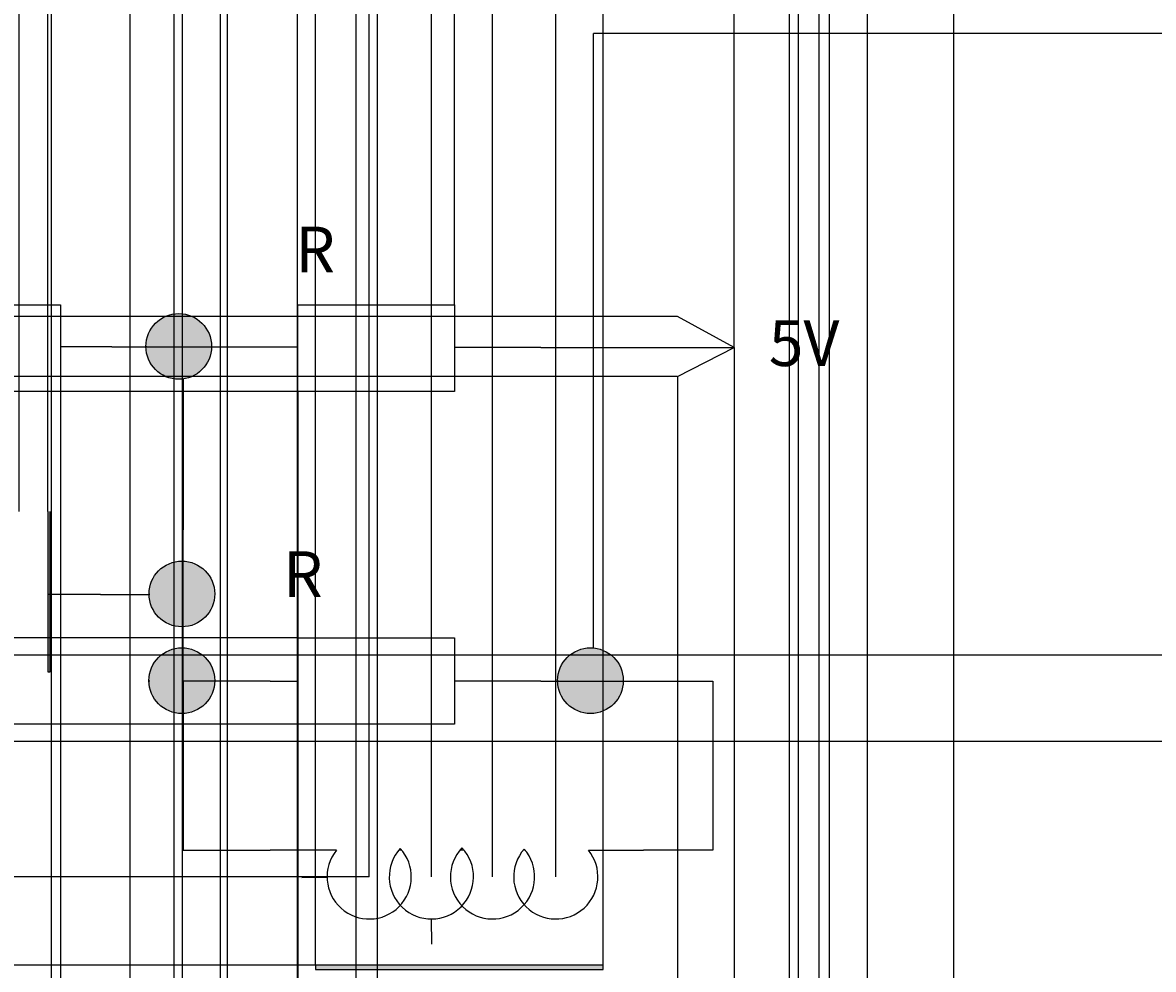
# Model space of a CAD drawing. Units: inches. Extents: x 35362 to 73946, y 43607 to 67532.
# Tile 127 of 134: x 52380 to 57838, y 46109 to 50677. Entities that reach past the tile are written whole.
import ezdxf

# ---------------------------------------------------------------- set-up
doc = ezdxf.new("R2010")
doc.units = ezdxf.units.IN
doc.header["$MEASUREMENT"] = 0
for name, color, linetype, lineweight in [('A-ANNO-DIMS', 2, 'Continuous', 18), ('E-ANNO-TEXT', 5, 'Continuous', 18), ('E-SYMB', 1, 'Continuous', 25), ('E-SYMB-PATT', 1, 'Continuous', 13), ('E-WIRE', 3, 'Continuous', 25)]:
    doc.layers.add(name, color=color, linetype=linetype, lineweight=lineweight)
doc.styles.get("Standard").update_dxf_attribs({"font": 'arial.ttf'})
doc.dimstyles.get("Standard").update_dxf_attribs({"dimtxt": 0.18, "dimasz": 0.18, "dimexe": 0.18, "dimexo": 0.0625, "dimgap": 0.09, "dimtad": 0, "dimtih": 1, "dimtoh": 1, "dimdec": 4, "dimzin": 0, "dimdsep": 46, "dimtxsty": 'Standard', "dimcen": 0.09, "dimadec": 0, "dimazin": 0, "dimtfac": 1, "dimtdec": 4, "dimtofl": 0, "dimtmove": 0, "dimatfit": 3, "dimfxl": 1, "dimtolj": 1, "dimtzin": 0, "dimarcsym": 0})

# ---------------------------------------------------------------- blocks, each defined once
blk = doc.blocks.new('CT-CORE')
for p, q in [((0, 1388), (0, 0)), ((20, 1388), (0, 1388)), ((20, 0), (20, 1388)), ((270.7, 1388), (270.7, 0)), ((290.7, 1388), (270.7, 1388)), ((290.7, 0), (290.7, 1388)), ((659, 1388), (659, 1014.6)), ((679, 1388), (659, 1388)), ((679, 1015.4), (679, 1388)), ((659, 544.4), (659, 0)), ((679, 0), (679, 543.5)), ((0, 0), (20, 0)), ((270.7, 0), (290.7, 0)), ((659, 0), (679, 0))]:
    blk.add_line(p, q)
blk.add_arc((679, 779.5), 235.9, 90, 270)
blk = doc.blocks.new('PWR-5V')
for p, q in [((149.8, 1350.9), (0, 1075.9)), ((149.8, 833.1), (149.8, 1350.9)), ((290, 1075.9), (149.8, 1350.9)), ((149.8, 416.3), (149.8, 833.1)), ((149.8, 416.3), (149.8, 0))]:
    blk.add_line(p, q)
blk = doc.blocks.new('*D5')
at = {"layer": 'A-ANNO-DIMS', "color": 0, "lineweight": -2, "transparency": 16777216}
for p, q in [((37121.9, 46919.3), (37121.9, 43606.7)), ((69871.5, 45449.8), (69871.5, 43606.7)), ((37122.1, 43606.9), (53496.3, 43606.9)), ((69871.3, 43606.9), (53497.2, 43606.9))]:
    blk.add_line(p, q, dxfattribs=at)
at = {"layer": 'A-ANNO-DIMS', "color": 0, "transparency": 16777216}
for points in [[(37122.1, 43606.9), (37122.1, 43606.8), (37121.9, 43606.9)], [(69871.3, 43606.9), (69871.3, 43606.8), (69871.5, 43606.9)]]:
    blk.add_solid(points, dxfattribs=at)
at = {"layer": 'Defpoints', "color": 0, "transparency": 16777216}
for p in [(37121.9, 46919.4), (69871.5, 45449.9), (69871.5, 43606.9)]:
    blk.add_point(p, dxfattribs=at)
at = {"layer": 'A-ANNO-DIMS', "color": 0, "transparency": 16777216, "insert": (53496.7, 43606.9), "char_height": 0.18, "attachment_point": 5}
blk.add_mtext('\\A1;32750', dxfattribs=at)
blk = doc.blocks.new('*D11')
at = {"layer": 'A-ANNO-DIMS', "color": 0, "lineweight": -2, "transparency": 16777216}
for p, q in [((47978.7, 56028.8), (47978.7, 43606.7)), ((53109.8, 56028.8), (53109.8, 43606.7)), ((47978.8, 43606.9), (50543.9, 43606.9)), ((53109.6, 43606.9), (50544.6, 43606.9))]:
    blk.add_line(p, q, dxfattribs=at)
at = {"layer": 'A-ANNO-DIMS', "color": 0, "transparency": 16777216}
for points in [[(47978.8, 43606.9), (47978.8, 43606.8), (47978.7, 43606.9)], [(53109.6, 43606.9), (53109.6, 43606.8), (53109.8, 43606.9)]]:
    blk.add_solid(points, dxfattribs=at)
at = {"layer": 'Defpoints', "color": 0, "transparency": 16777216}
for p in [(47978.7, 56028.8), (53109.8, 56028.8), (53109.8, 43606.9)]:
    blk.add_point(p, dxfattribs=at)
at = {"layer": 'A-ANNO-DIMS', "color": 0, "transparency": 16777216, "insert": (50544.2, 43606.9), "char_height": 0.18, "attachment_point": 5}
blk.add_mtext('\\A1;5131', dxfattribs=at)
blk = doc.blocks.new('*D23')
at = {"layer": 'A-ANNO-DIMS', "color": 0, "lineweight": -2, "transparency": 16777216}
for p, q in [((53727.6, 46552.2), (53849.4, 46553.3)), ((54052.8, 46555.3), (54053, 46555.3)), ((54052.9, 46555.2), (54052.9, 46555.4))]:
    blk.add_line(p, q, dxfattribs=at)
at = {"layer": 'A-ANNO-DIMS', "color": 0, "transparency": 16777216}
blk.add_solid([(53849.4, 46553.4), (53849.4, 46553.3), (53849.6, 46553.3)], dxfattribs=at)
at = {"layer": 'Defpoints', "color": 0, "transparency": 16777216}
for p in [(53849.6, 46553.3), (54052.9, 46555.3)]:
    blk.add_point(p, dxfattribs=at)
at = {"layer": 'A-ANNO-DIMS', "color": 0, "transparency": 16777216, "insert": (53726.8, 46552.2), "char_height": 0.18, "attachment_point": 5}
blk.add_mtext('\\A1;20X R203.33', dxfattribs=at)
blk = doc.blocks.new('*D39')
at = {"layer": 'A-ANNO-DIMS', "color": 0, "lineweight": -2, "transparency": 16777216}
for p, q in [((53793.6, 46128.9), (53793.6, 67531.7)), ((53793.8, 67531.5), (54487.2, 67531.5)), ((55181.5, 67531.5), (54488.1, 67531.5)), ((55181.6, 46128.9), (55181.6, 67531.7))]:
    blk.add_line(p, q, dxfattribs=at)
at = {"layer": 'A-ANNO-DIMS', "color": 0, "transparency": 16777216}
for points in [[(53793.8, 67531.5), (53793.8, 67531.5), (53793.6, 67531.5)], [(55181.5, 67531.5), (55181.5, 67531.5), (55181.6, 67531.5)]]:
    blk.add_solid(points, dxfattribs=at)
at = {"layer": 'Defpoints', "color": 0, "transparency": 16777216}
for p in [(55181.6, 67531.5), (53793.6, 46128.9), (55181.6, 46128.9)]:
    blk.add_point(p, dxfattribs=at)
at = {"layer": 'A-ANNO-DIMS', "color": 0, "transparency": 16777216, "insert": (54487.6, 67531.5), "char_height": 0.18, "attachment_point": 5}
blk.add_mtext('\\A1;1388.0', dxfattribs=at)
blk = doc.blocks.new('*D40')
at = {"layer": 'A-ANNO-DIMS', "color": 0, "lineweight": -2, "transparency": 16777216}
for p, q in [((56873.5, 53351.5), (35361.8, 53351.5)), ((35361.9, 53351.3), (35361.9, 51333.3)), ((35361.9, 49314.8), (35361.9, 51332.9)), ((51806.5, 49314.7), (35361.8, 49314.7))]:
    blk.add_line(p, q, dxfattribs=at)
at = {"layer": 'A-ANNO-DIMS', "color": 0, "transparency": 16777216}
for points in [[(35361.9, 53351.3), (35362, 53351.3), (35361.9, 53351.5)], [(35361.9, 49314.8), (35362, 49314.8), (35361.9, 49314.7)]]:
    blk.add_solid(points, dxfattribs=at)
at = {"layer": 'Defpoints', "color": 0, "transparency": 16777216}
for p in [(35361.9, 53351.5), (56873.6, 53351.5), (51806.5, 49314.7)]:
    blk.add_point(p, dxfattribs=at)
at = {"layer": 'A-ANNO-DIMS', "color": 0, "transparency": 16777216, "insert": (35361.9, 51333.1), "char_height": 0.18, "attachment_point": 5}
blk.add_mtext('\\A1;4036.9', dxfattribs=at)
blk = doc.blocks.new('*D43')
at = {"layer": 'A-ANNO-DIMS', "color": 0, "lineweight": -2, "transparency": 16777216}
for p, q in [((62004.7, 47625.2), (35361.8, 47625.2)), ((35361.9, 47625), (35361.9, 47416.9)), ((35361.9, 47208.4), (35361.9, 47416.5)), ((62004.7, 47208.2), (35361.8, 47208.2))]:
    blk.add_line(p, q, dxfattribs=at)
at = {"layer": 'A-ANNO-DIMS', "color": 0, "transparency": 16777216}
for points in [[(35361.9, 47625), (35362, 47625), (35361.9, 47625.2)], [(35361.9, 47208.4), (35362, 47208.4), (35361.9, 47208.2)]]:
    blk.add_solid(points, dxfattribs=at)
at = {"layer": 'Defpoints', "color": 0, "transparency": 16777216}
for p in [(62004.7, 47625.2), (35361.9, 47208.2), (62004.7, 47208.2)]:
    blk.add_point(p, dxfattribs=at)
at = {"layer": 'A-ANNO-DIMS', "color": 0, "transparency": 16777216, "insert": (35361.9, 47416.7), "char_height": 0.18, "attachment_point": 5}
blk.add_mtext('\\A1;416.9', dxfattribs=at)
blk = doc.blocks.new('*D44')
at = {"layer": 'A-ANNO-DIMS', "color": 0, "lineweight": -2, "transparency": 16777216}
for p, q in [((52517.8, 64828.5), (52517.8, 43606.7)), ((54090.8, 64828.5), (54090.8, 43606.7)), ((52518, 43606.9), (53303.8, 43606.9)), ((54090.6, 43606.9), (53304.7, 43606.9))]:
    blk.add_line(p, q, dxfattribs=at)
at = {"layer": 'A-ANNO-DIMS', "color": 0, "transparency": 16777216}
for points in [[(52518, 43606.9), (52518, 43606.8), (52517.8, 43606.9)], [(54090.6, 43606.9), (54090.6, 43606.8), (54090.8, 43606.9)]]:
    blk.add_solid(points, dxfattribs=at)
at = {"layer": 'Defpoints', "color": 0, "transparency": 16777216}
for p in [(52517.8, 64828.6), (54090.8, 64828.6), (54090.8, 43606.9)]:
    blk.add_point(p, dxfattribs=at)
at = {"layer": 'A-ANNO-DIMS', "color": 0, "transparency": 16777216, "insert": (53304.3, 43606.9), "char_height": 0.18, "attachment_point": 5}
blk.add_mtext('\\A1;1573.0', dxfattribs=at)
blk = doc.blocks.new('*D49')
at = {"layer": 'A-ANNO-DIMS', "color": 0, "lineweight": -2, "transparency": 16777216}
for p, q in [((56457.3, 54249.8), (56457.3, 43606.7)), ((56873.6, 54249.8), (56873.6, 43606.7)), ((56457.5, 43606.9), (56665, 43606.9)), ((56873.4, 43606.9), (56665.8, 43606.9))]:
    blk.add_line(p, q, dxfattribs=at)
at = {"layer": 'A-ANNO-DIMS', "color": 0, "transparency": 16777216}
for points in [[(56457.5, 43606.9), (56457.5, 43606.8), (56457.3, 43606.9)], [(56873.4, 43606.9), (56873.4, 43606.8), (56873.6, 43606.9)]]:
    blk.add_solid(points, dxfattribs=at)
at = {"layer": 'Defpoints', "color": 0, "transparency": 16777216}
for p in [(56457.3, 54249.8), (56873.6, 54249.8), (56873.6, 43606.9)]:
    blk.add_point(p, dxfattribs=at)
at = {"layer": 'A-ANNO-DIMS', "color": 0, "transparency": 16777216, "insert": (56665.4, 43606.9), "char_height": 0.18, "attachment_point": 5}
blk.add_mtext('\\A1;416.3', dxfattribs=at)
blk = doc.blocks.new('*D53')
at = {"layer": 'A-ANNO-DIMS', "color": 0, "lineweight": -2, "transparency": 16777216}
for p, q in [((56873.6, 53351.5), (56873.6, 43606.7)), ((58224.8, 52935.2), (58224.8, 43606.7)), ((56873.8, 43606.9), (57548.7, 43606.9)), ((58224.6, 43606.9), (57549.6, 43606.9))]:
    blk.add_line(p, q, dxfattribs=at)
at = {"layer": 'A-ANNO-DIMS', "color": 0, "transparency": 16777216}
for points in [[(56873.8, 43606.9), (56873.8, 43606.8), (56873.6, 43606.9)], [(58224.6, 43606.9), (58224.6, 43606.8), (58224.8, 43606.9)]]:
    blk.add_solid(points, dxfattribs=at)
at = {"layer": 'Defpoints', "color": 0, "transparency": 16777216}
for p in [(56873.6, 53351.5), (58224.8, 52935.2), (58224.8, 43606.9)]:
    blk.add_point(p, dxfattribs=at)
at = {"layer": 'A-ANNO-DIMS', "color": 0, "transparency": 16777216, "insert": (57549.2, 43606.9), "char_height": 0.18, "attachment_point": 5}
blk.add_mtext('\\A1;1351.2', dxfattribs=at)
blk = doc.blocks.new('*D63')
at = {"layer": 'A-ANNO-DIMS', "color": 0, "lineweight": -2, "transparency": 16777216}
for p, q in [((53727.6, 46552.2), (53849.4, 46553.3)), ((54052.8, 46555.3), (54053, 46555.3)), ((54052.9, 46555.2), (54052.9, 46555.4))]:
    blk.add_line(p, q, dxfattribs=at)
at = {"layer": 'A-ANNO-DIMS', "color": 0, "transparency": 16777216}
blk.add_solid([(53849.4, 46553.4), (53849.4, 46553.3), (53849.6, 46553.3)], dxfattribs=at)
at = {"layer": 'Defpoints', "color": 0, "transparency": 16777216}
for p in [(53849.6, 46553.3), (54052.9, 46555.3)]:
    blk.add_point(p, dxfattribs=at)
at = {"layer": 'A-ANNO-DIMS', "color": 0, "transparency": 16777216, "insert": (53726.8, 46552.2), "char_height": 0.18, "attachment_point": 5}
blk.add_mtext('\\A1;20X R203.33', dxfattribs=at)
blk = doc.blocks.new('*D67')
at = {"layer": 'A-ANNO-DIMS', "color": 0, "lineweight": -2, "transparency": 16777216}
for p, q in [((56873.5, 53351.5), (35361.8, 53351.5)), ((35361.9, 53351.3), (35361.9, 49400.9)), ((35361.9, 45450.1), (35361.9, 49400.5)), ((53793.6, 45449.9), (35361.8, 45449.9))]:
    blk.add_line(p, q, dxfattribs=at)
at = {"layer": 'A-ANNO-DIMS', "color": 0, "transparency": 16777216}
for points in [[(35361.9, 53351.3), (35362, 53351.3), (35361.9, 53351.5)], [(35361.9, 45450.1), (35362, 45450.1), (35361.9, 45449.9)]]:
    blk.add_solid(points, dxfattribs=at)
at = {"layer": 'Defpoints', "color": 0, "transparency": 16777216}
for p in [(35361.9, 53351.5), (56873.6, 53351.5), (53793.6, 45449.9)]:
    blk.add_point(p, dxfattribs=at)
at = {"layer": 'A-ANNO-DIMS', "color": 0, "transparency": 16777216, "insert": (35361.9, 49400.7), "char_height": 0.18, "attachment_point": 5}
blk.add_mtext('\\A1;7901.6', dxfattribs=at)
blk = doc.blocks.new('*D76')
at = {"layer": 'A-ANNO-DIMS', "color": 0, "lineweight": -2, "transparency": 16777216}
for p, q in [((54052.8, 46555.3), (35361.8, 46555.3)), ((35361.9, 46555.1), (35361.9, 46342.3)), ((35361.9, 46129.1), (35361.9, 46341.9)), ((53793.6, 46128.9), (35361.8, 46128.9))]:
    blk.add_line(p, q, dxfattribs=at)
at = {"layer": 'A-ANNO-DIMS', "color": 0, "transparency": 16777216}
for points in [[(35361.9, 46555.1), (35362, 46555.1), (35361.9, 46555.3)], [(35361.9, 46129.1), (35362, 46129.1), (35361.9, 46128.9)]]:
    blk.add_solid(points, dxfattribs=at)
at = {"layer": 'Defpoints', "color": 0, "transparency": 16777216}
for p in [(35361.9, 46555.3), (54052.9, 46555.3), (53793.6, 46128.9)]:
    blk.add_point(p, dxfattribs=at)
at = {"layer": 'A-ANNO-DIMS', "color": 0, "transparency": 16777216, "insert": (35361.9, 46342.1), "char_height": 0.18, "attachment_point": 5}
blk.add_mtext('\\A1;426.4', dxfattribs=at)
blk = doc.blocks.new('*D77')
at = {"layer": 'A-ANNO-DIMS', "color": 0, "lineweight": -2, "transparency": 16777216}
for p, q in [((53793.6, 46128.9), (53793.6, 67531.7)), ((53793.8, 67531.5), (53922.8, 67531.5)), ((54052.7, 67531.5), (53923.7, 67531.5)), ((54052.9, 46555.4), (54052.9, 67531.7))]:
    blk.add_line(p, q, dxfattribs=at)
at = {"layer": 'A-ANNO-DIMS', "color": 0, "transparency": 16777216}
for points in [[(53793.8, 67531.5), (53793.8, 67531.5), (53793.6, 67531.5)], [(54052.7, 67531.5), (54052.7, 67531.5), (54052.9, 67531.5)]]:
    blk.add_solid(points, dxfattribs=at)
at = {"layer": 'Defpoints', "color": 0, "transparency": 16777216}
for p in [(54052.9, 67531.5), (54052.9, 46555.3), (53793.6, 46128.9)]:
    blk.add_point(p, dxfattribs=at)
at = {"layer": 'A-ANNO-DIMS', "color": 0, "transparency": 16777216, "insert": (53923.3, 67531.5), "char_height": 0.18, "attachment_point": 5}
blk.add_mtext('\\A1;259.26', dxfattribs=at)
blk = doc.blocks.new('*D78')
at = {"layer": 'A-ANNO-DIMS', "color": 0, "lineweight": -2, "transparency": 16777216}
for p, q in [((54052.9, 46555.4), (54052.9, 67531.7)), ((54053.1, 67531.5), (54202.6, 67531.5)), ((54352.9, 67531.5), (54203.4, 67531.5)), ((54353.1, 46555.4), (54353.1, 67531.7))]:
    blk.add_line(p, q, dxfattribs=at)
at = {"layer": 'A-ANNO-DIMS', "color": 0, "transparency": 16777216}
for points in [[(54053.1, 67531.5), (54053.1, 67531.5), (54052.9, 67531.5)], [(54352.9, 67531.5), (54352.9, 67531.5), (54353.1, 67531.5)]]:
    blk.add_solid(points, dxfattribs=at)
at = {"layer": 'Defpoints', "color": 0, "transparency": 16777216}
for p in [(54353.1, 67531.5), (54052.9, 46555.3), (54353.1, 46555.3)]:
    blk.add_point(p, dxfattribs=at)
at = {"layer": 'A-ANNO-DIMS', "color": 0, "transparency": 16777216, "insert": (54203, 67531.5), "char_height": 0.18, "attachment_point": 5}
blk.add_mtext('\\A1;300.2', dxfattribs=at)
blk = doc.blocks.new('*D79')
at = {"layer": 'A-ANNO-DIMS', "color": 0, "lineweight": -2, "transparency": 16777216}
for p, q in [((54353.1, 46555.4), (54353.1, 67531.7)), ((54353.3, 67531.5), (54500.2, 67531.5)), ((54648, 67531.5), (54501, 67531.5)), ((54648.2, 46555.4), (54648.2, 67531.7))]:
    blk.add_line(p, q, dxfattribs=at)
at = {"layer": 'A-ANNO-DIMS', "color": 0, "transparency": 16777216}
for points in [[(54353.3, 67531.5), (54353.3, 67531.5), (54353.1, 67531.5)], [(54648, 67531.5), (54648, 67531.5), (54648.2, 67531.5)]]:
    blk.add_solid(points, dxfattribs=at)
at = {"layer": 'Defpoints', "color": 0, "transparency": 16777216}
for p in [(54648.2, 67531.5), (54353.1, 46555.3), (54648.2, 46555.3)]:
    blk.add_point(p, dxfattribs=at)
at = {"layer": 'A-ANNO-DIMS', "color": 0, "transparency": 16777216, "insert": (54500.6, 67531.5), "char_height": 0.18, "attachment_point": 5}
blk.add_mtext('\\A1;295.1', dxfattribs=at)
blk = doc.blocks.new('*D80')
at = {"layer": 'A-ANNO-DIMS', "color": 0, "lineweight": -2, "transparency": 16777216}
for p, q in [((54648.2, 46555.4), (54648.2, 67531.7)), ((54648.4, 67531.5), (54800.3, 67531.5)), ((54953.3, 67531.5), (54801.3, 67531.5)), ((54953.4, 46555.4), (54953.4, 67531.7))]:
    blk.add_line(p, q, dxfattribs=at)
at = {"layer": 'A-ANNO-DIMS', "color": 0, "transparency": 16777216}
for points in [[(54648.4, 67531.5), (54648.4, 67531.5), (54648.2, 67531.5)], [(54953.3, 67531.5), (54953.3, 67531.5), (54953.4, 67531.5)]]:
    blk.add_solid(points, dxfattribs=at)
at = {"layer": 'Defpoints', "color": 0, "transparency": 16777216}
for p in [(54953.4, 67531.5), (54648.2, 46555.3), (54953.4, 46555.3)]:
    blk.add_point(p, dxfattribs=at)
at = {"layer": 'A-ANNO-DIMS', "color": 0, "transparency": 16777216, "insert": (54800.8, 67531.5), "char_height": 0.18, "attachment_point": 5}
blk.add_mtext('\\A1;305.27', dxfattribs=at)
blk = doc.blocks.new('*D82')
at = {"layer": 'A-ANNO-DIMS', "color": 0, "lineweight": -2, "transparency": 16777216}
for p, q in [((54464.4, 49314.7), (54464.4, 67531.7)), ((54464.6, 67531.5), (55139.4, 67531.5)), ((55815.1, 67531.5), (55140.3, 67531.5)), ((55815.3, 49110.2), (55815.3, 67531.7))]:
    blk.add_line(p, q, dxfattribs=at)
at = {"layer": 'A-ANNO-DIMS', "color": 0, "transparency": 16777216}
for points in [[(54464.6, 67531.5), (54464.6, 67531.5), (54464.4, 67531.5)], [(55815.1, 67531.5), (55815.1, 67531.5), (55815.3, 67531.5)]]:
    blk.add_solid(points, dxfattribs=at)
at = {"layer": 'Defpoints', "color": 0, "transparency": 16777216}
for p in [(55815.3, 67531.5), (54464.4, 49314.7), (55815.3, 49110.1)]:
    blk.add_point(p, dxfattribs=at)
at = {"layer": 'A-ANNO-DIMS', "color": 0, "transparency": 16777216, "insert": (55139.9, 67531.5), "char_height": 0.18, "attachment_point": 5}
blk.add_mtext('\\A1;1350.9', dxfattribs=at)
blk = doc.blocks.new('*D83')
at = {"layer": 'A-ANNO-DIMS', "color": 0, "lineweight": -2, "transparency": 16777216}
for p, q in [((55815.3, 49110), (55815.3, 43606.7)), ((55540.3, 48969.9), (55540.3, 43606.7)), ((55540.5, 43606.9), (55677.4, 43606.9)), ((55815.1, 43606.9), (55678.2, 43606.9))]:
    blk.add_line(p, q, dxfattribs=at)
at = {"layer": 'A-ANNO-DIMS', "color": 0, "transparency": 16777216}
for points in [[(55540.5, 43606.9), (55540.5, 43606.8), (55540.3, 43606.9)], [(55815.1, 43606.9), (55815.1, 43606.8), (55815.3, 43606.9)]]:
    blk.add_solid(points, dxfattribs=at)
at = {"layer": 'Defpoints', "color": 0, "transparency": 16777216}
for p in [(55815.3, 49110.1), (55540.3, 48970), (55815.3, 43606.9)]:
    blk.add_point(p, dxfattribs=at)
at = {"layer": 'A-ANNO-DIMS', "color": 0, "transparency": 16777216, "insert": (55677.8, 43606.9), "char_height": 0.18, "attachment_point": 5}
blk.add_mtext('\\A1;275.0', dxfattribs=at)
blk = doc.blocks.new('*D84')
at = {"layer": 'A-ANNO-DIMS', "color": 0, "lineweight": -2, "transparency": 16777216}
for p, q in [((55540.2, 49259.9), (35361.8, 49259.9)), ((35361.9, 49259.8), (35361.9, 49115.1)), ((35361.9, 48970.2), (35361.9, 49114.8)), ((55540.2, 48970), (35361.8, 48970))]:
    blk.add_line(p, q, dxfattribs=at)
at = {"layer": 'A-ANNO-DIMS', "color": 0, "transparency": 16777216}
for points in [[(35361.9, 49259.8), (35362, 49259.8), (35361.9, 49259.9)], [(35361.9, 48970.2), (35362, 48970.2), (35361.9, 48970)]]:
    blk.add_solid(points, dxfattribs=at)
at = {"layer": 'Defpoints', "color": 0, "transparency": 16777216}
for p in [(35361.9, 49259.9), (55540.3, 49259.9), (55540.3, 48970)]:
    blk.add_point(p, dxfattribs=at)
at = {"layer": 'A-ANNO-DIMS', "color": 0, "transparency": 16777216, "insert": (35361.9, 49115), "char_height": 0.18, "attachment_point": 5}
blk.add_mtext('\\A1;289.96', dxfattribs=at)
blk = doc.blocks.new('*D88')
at = {"layer": 'A-ANNO-DIMS', "color": 0, "lineweight": -2, "transparency": 16777216}
for p, q in [((52362.6, 48318.3), (52362.6, 67531.7)), ((52362.7, 67531.5), (52432.1, 67531.5)), ((52502.2, 67531.5), (52432.8, 67531.5)), ((52502.4, 48318.3), (52502.4, 67531.7))]:
    blk.add_line(p, q, dxfattribs=at)
at = {"layer": 'A-ANNO-DIMS', "color": 0, "transparency": 16777216}
for points in [[(52362.7, 67531.5), (52362.7, 67531.5), (52362.6, 67531.5)], [(52502.2, 67531.5), (52502.2, 67531.5), (52502.4, 67531.5)]]:
    blk.add_solid(points, dxfattribs=at)
at = {"layer": 'Defpoints', "color": 0, "transparency": 16777216}
for p in [(52502.4, 67531.5), (52362.6, 48318.3), (52502.4, 48318.3)]:
    blk.add_point(p, dxfattribs=at)
at = {"layer": 'A-ANNO-DIMS', "color": 0, "transparency": 16777216, "insert": (52432.5, 67531.5), "char_height": 0.18, "attachment_point": 5}
blk.add_mtext('\\A1;139.8', dxfattribs=at)
blk = doc.blocks.new('*D89')
at = {"layer": 'A-ANNO-DIMS', "color": 0, "lineweight": -2, "transparency": 16777216}
for p, q in [((53707.7, 48897.7), (35361.8, 48897.7)), ((35361.9, 48897.6), (35361.9, 48303.2)), ((35361.9, 47708.4), (35361.9, 48302.8)), ((53707.7, 47708.2), (35361.8, 47708.2))]:
    blk.add_line(p, q, dxfattribs=at)
at = {"layer": 'A-ANNO-DIMS', "color": 0, "transparency": 16777216}
for points in [[(35361.9, 48897.6), (35362, 48897.6), (35361.9, 48897.7)], [(35361.9, 47708.4), (35362, 47708.4), (35361.9, 47708.2)]]:
    blk.add_solid(points, dxfattribs=at)
at = {"layer": 'Defpoints', "color": 0, "transparency": 16777216}
for p in [(53707.8, 48897.7), (35361.9, 47708.2), (53707.8, 47708.2)]:
    blk.add_point(p, dxfattribs=at)
at = {"layer": 'A-ANNO-DIMS', "color": 0, "transparency": 16777216, "insert": (35361.9, 48303), "char_height": 0.18, "attachment_point": 5}
blk.add_mtext('\\A1;1189.5', dxfattribs=at)
blk = doc.blocks.new('*D90')
at = {"layer": 'A-ANNO-DIMS', "color": 0, "lineweight": -2, "transparency": 16777216}
for p, q in [((53707.7, 47291.3), (35361.8, 47291.3)), ((35361.9, 47291.1), (35361.9, 46710.3)), ((35361.9, 46129.1), (35361.9, 46709.9)), ((53793.6, 46128.9), (35361.8, 46128.9))]:
    blk.add_line(p, q, dxfattribs=at)
at = {"layer": 'A-ANNO-DIMS', "color": 0, "transparency": 16777216}
for points in [[(35361.9, 47291.1), (35362, 47291.1), (35361.9, 47291.3)], [(35361.9, 46129.1), (35362, 46129.1), (35361.9, 46128.9)]]:
    blk.add_solid(points, dxfattribs=at)
at = {"layer": 'Defpoints', "color": 0, "transparency": 16777216}
for p in [(53707.8, 47291.3), (35361.9, 46128.9), (53793.6, 46128.9)]:
    blk.add_point(p, dxfattribs=at)
at = {"layer": 'A-ANNO-DIMS', "color": 0, "transparency": 16777216, "insert": (35361.9, 46710.1), "char_height": 0.18, "attachment_point": 5}
blk.add_mtext('\\A1;1162.4', dxfattribs=at)
blk = doc.blocks.new('*D91')
at = {"layer": 'A-ANNO-DIMS', "color": 0, "lineweight": -2, "transparency": 16777216}
for p, q in [((52563.1, 48897.7), (52563.1, 43606.7)), ((53707.8, 48897.7), (53707.8, 43606.7)), ((52563.3, 43606.9), (53135, 43606.9)), ((53707.6, 43606.9), (53135.9, 43606.9))]:
    blk.add_line(p, q, dxfattribs=at)
at = {"layer": 'A-ANNO-DIMS', "color": 0, "transparency": 16777216}
for points in [[(52563.3, 43606.9), (52563.3, 43606.8), (52563.1, 43606.9)], [(53707.6, 43606.9), (53707.6, 43606.8), (53707.8, 43606.9)]]:
    blk.add_solid(points, dxfattribs=at)
at = {"layer": 'Defpoints', "color": 0, "transparency": 16777216}
for p in [(52563.1, 48897.7), (53707.8, 48897.7), (53707.8, 43606.9)]:
    blk.add_point(p, dxfattribs=at)
at = {"layer": 'A-ANNO-DIMS', "color": 0, "transparency": 16777216, "insert": (53135.5, 43606.9), "char_height": 0.18, "attachment_point": 5}
blk.add_mtext('\\A1;1144.6', dxfattribs=at)
blk = doc.blocks.new('*D96')
at = {"layer": 'A-ANNO-DIMS', "color": 0, "lineweight": -2, "transparency": 16777216}
for p, q in [((53366.8, 64997.6), (53366.8, 43606.7)), ((53988.6, 64997.6), (53988.6, 43606.7)), ((53366.9, 43606.9), (53677.3, 43606.9)), ((53988.4, 43606.9), (53678.1, 43606.9))]:
    blk.add_line(p, q, dxfattribs=at)
at = {"layer": 'A-ANNO-DIMS', "color": 0, "transparency": 16777216}
for points in [[(53366.9, 43606.9), (53366.9, 43606.8), (53366.8, 43606.9)], [(53988.4, 43606.9), (53988.4, 43606.8), (53988.6, 43606.9)]]:
    blk.add_solid(points, dxfattribs=at)
at = {"layer": 'Defpoints', "color": 0, "transparency": 16777216}
for p in [(53366.8, 64997.7), (53988.6, 64997.7), (53988.6, 43606.9)]:
    blk.add_point(p, dxfattribs=at)
at = {"layer": 'A-ANNO-DIMS', "color": 0, "transparency": 16777216, "insert": (53677.7, 43606.9), "char_height": 0.18, "attachment_point": 5}
blk.add_mtext('\\A1;621.8', dxfattribs=at)
blk = doc.blocks.new('*D99')
at = {"layer": 'A-ANNO-DIMS', "color": 0, "lineweight": -2, "transparency": 16777216}
for p, q in [((52897.5, 65291.5), (52897.5, 43606.7)), ((52517.8, 64828.5), (52517.8, 43606.7)), ((52518, 43606.9), (52707.2, 43606.9)), ((52897.3, 43606.9), (52708, 43606.9))]:
    blk.add_line(p, q, dxfattribs=at)
at = {"layer": 'A-ANNO-DIMS', "color": 0, "transparency": 16777216}
for points in [[(52518, 43606.9), (52518, 43606.8), (52517.8, 43606.9)], [(52897.3, 43606.9), (52897.3, 43606.8), (52897.5, 43606.9)]]:
    blk.add_solid(points, dxfattribs=at)
at = {"layer": 'Defpoints', "color": 0, "transparency": 16777216}
for p in [(52897.5, 65291.6), (52517.8, 64828.6), (52897.5, 43606.9)]:
    blk.add_point(p, dxfattribs=at)
at = {"layer": 'A-ANNO-DIMS', "color": 0, "transparency": 16777216, "insert": (52707.6, 43606.9), "char_height": 0.18, "attachment_point": 5}
blk.add_mtext('\\A1;379.7', dxfattribs=at)
blk = doc.blocks.new('*D100')
at = {"layer": 'A-ANNO-DIMS', "color": 0, "lineweight": -2, "transparency": 16777216}
for p, q in [((52897.5, 65291.5), (52897.5, 43606.7)), ((53150.7, 64926.1), (53150.7, 43606.7)), ((52897.7, 43606.9), (53023.7, 43606.9)), ((53150.5, 43606.9), (53024.5, 43606.9))]:
    blk.add_line(p, q, dxfattribs=at)
at = {"layer": 'A-ANNO-DIMS', "color": 0, "transparency": 16777216}
for points in [[(52897.7, 43606.9), (52897.7, 43606.8), (52897.5, 43606.9)], [(53150.5, 43606.9), (53150.5, 43606.8), (53150.7, 43606.9)]]:
    blk.add_solid(points, dxfattribs=at)
at = {"layer": 'Defpoints', "color": 0, "transparency": 16777216}
for p in [(52897.5, 65291.6), (53150.7, 64926.1), (53150.7, 43606.9)]:
    blk.add_point(p, dxfattribs=at)
at = {"layer": 'A-ANNO-DIMS', "color": 0, "transparency": 16777216, "insert": (53024.1, 43606.9), "char_height": 0.18, "attachment_point": 5}
blk.add_mtext('\\A1;253.2', dxfattribs=at)
blk = doc.blocks.new('*D102')
at = {"layer": 'A-ANNO-DIMS', "color": 0, "lineweight": -2, "transparency": 16777216}
for p, q in [((56080.5, 63694.7), (56080.5, 43606.7)), ((56272.5, 63696.8), (56272.5, 43606.7)), ((56080.7, 43606.9), (56176, 43606.9)), ((56272.3, 43606.9), (56176.9, 43606.9))]:
    blk.add_line(p, q, dxfattribs=at)
at = {"layer": 'A-ANNO-DIMS', "color": 0, "transparency": 16777216}
for points in [[(56080.7, 43606.9), (56080.7, 43606.8), (56080.5, 43606.9)], [(56272.3, 43606.9), (56272.3, 43606.8), (56272.5, 43606.9)]]:
    blk.add_solid(points, dxfattribs=at)
at = {"layer": 'Defpoints', "color": 0, "transparency": 16777216}
for p in [(56080.5, 63694.8), (56272.5, 63696.9), (56272.5, 43606.9)]:
    blk.add_point(p, dxfattribs=at)
at = {"layer": 'A-ANNO-DIMS', "color": 0, "transparency": 16777216, "insert": (56176.5, 43606.9), "char_height": 0.18, "attachment_point": 5}
blk.add_mtext('\\A1;191.98', dxfattribs=at)
blk = doc.blocks.new('*D104')
at = {"layer": 'A-ANNO-DIMS', "color": 0, "lineweight": -2, "transparency": 16777216}
for p, q in [((56123.2, 63318.1), (56123.2, 43606.7)), ((56223, 63318.1), (56223, 43606.7)), ((56123.4, 43606.9), (56172.7, 43606.9)), ((56222.8, 43606.9), (56173.5, 43606.9))]:
    blk.add_line(p, q, dxfattribs=at)
at = {"layer": 'A-ANNO-DIMS', "color": 0, "transparency": 16777216}
for points in [[(56123.4, 43606.9), (56123.4, 43606.8), (56123.2, 43606.9)], [(56222.8, 43606.9), (56222.8, 43606.8), (56223, 43606.9)]]:
    blk.add_solid(points, dxfattribs=at)
at = {"layer": 'Defpoints', "color": 0, "transparency": 16777216}
for p in [(56123.2, 63318.1), (56223, 63318.1), (56223, 43606.9)]:
    blk.add_point(p, dxfattribs=at)
at = {"layer": 'A-ANNO-DIMS', "color": 0, "transparency": 16777216, "insert": (56173.1, 43606.9), "char_height": 0.18, "attachment_point": 5}
blk.add_mtext('\\A1;99.74', dxfattribs=at)
blk = doc.blocks.new('*D112')
at = {"layer": 'A-ANNO-DIMS', "color": 0, "lineweight": -2, "transparency": 16777216}
for p, q in [((53332.8, 60113.4), (53332.8, 43606.7)), ((53705.4, 60126.2), (53705.4, 43606.7)), ((53332.9, 43606.9), (53518.7, 43606.9)), ((53705.2, 43606.9), (53519.5, 43606.9))]:
    blk.add_line(p, q, dxfattribs=at)
at = {"layer": 'A-ANNO-DIMS', "color": 0, "transparency": 16777216}
for points in [[(53332.9, 43606.9), (53332.9, 43606.8), (53332.8, 43606.9)], [(53705.2, 43606.9), (53705.2, 43606.8), (53705.4, 43606.9)]]:
    blk.add_solid(points, dxfattribs=at)
at = {"layer": 'Defpoints', "color": 0, "transparency": 16777216}
for p in [(53332.8, 60113.5), (53705.4, 60126.3), (53705.4, 43606.9)]:
    blk.add_point(p, dxfattribs=at)
at = {"layer": 'A-ANNO-DIMS', "color": 0, "transparency": 16777216, "insert": (53519.1, 43606.9), "char_height": 0.18, "attachment_point": 5}
blk.add_mtext('\\A1;372.6', dxfattribs=at)
blk = doc.blocks.new('*D114')
at = {"layer": 'A-ANNO-DIMS', "color": 0, "lineweight": -2, "transparency": 16777216}
for p, q in [((54353, 46555.3), (54353.2, 46555.3)), ((54353.1, 46555.2), (54353.1, 46555.4)), ((54354.6, 46230), (54354, 46351.8)), ((54354.7, 46230), (54354.6, 46230))]:
    blk.add_line(p, q, dxfattribs=at)
at = {"layer": 'A-ANNO-DIMS', "color": 0, "transparency": 16777216}
blk.add_solid([(54354, 46351.8), (54354, 46351.8), (54354, 46352)], dxfattribs=at)
at = {"layer": 'Defpoints', "color": 0, "transparency": 16777216}
for p in [(54353.1, 46555.3), (54354, 46352)]:
    blk.add_point(p, dxfattribs=at)
at = {"layer": 'A-ANNO-DIMS', "color": 0, "transparency": 16777216, "insert": (54355.5, 46230), "char_height": 0.18, "attachment_point": 5}
blk.add_mtext('\\A1;20X R203.33', dxfattribs=at)

msp = doc.modelspace()

# ---------------------------------------------------------------- hatches: boundary and pattern name
at = {"layer": 'E-SYMB-PATT'}
h = msp.add_hatch(color=256, dxfattribs=at)
h.dxf.hatch_style = 1
h.paths.add_polyline_path([(53292.156, 49112.547, 0.41839319), (53133.566, 49273.413, 0.41839319), (52974.976, 49112.547)])
h.paths.add_polyline_path([(53292.156, 49112.547), (52974.976, 49112.547, 0.41004625), (53133.566, 48956.201, 0.41004625)])
h = msp.add_hatch(color=256, dxfattribs=at)
h.dxf.hatch_style = 1
h.paths.add_polyline_path([(52502.363, 47544.134), (52513.518, 47544.134), (52513.518, 48318.269), (52502.363, 48318.269)])
h = msp.add_hatch(color=256, dxfattribs=at)
h.dxf.hatch_style = 1
h.paths.add_polyline_path([(53307.371, 47918.089, 0.41839319), (53148.782, 48078.955, 0.41839319), (52990.192, 47918.089)])
h.paths.add_polyline_path([(53307.371, 47918.089), (52990.192, 47918.089, 0.41004625), (53148.782, 47761.743, 0.41004625)])
h = msp.add_hatch(color=256, dxfattribs=at)
h.dxf.hatch_style = 1
h.paths.add_polyline_path([(53307.086, 47499.735, 0.41839319), (53148.496, 47660.601, 0.41839319), (52989.906, 47499.735)])
h.paths.add_polyline_path([(53307.086, 47499.735), (52989.906, 47499.735, 0.41004625), (53148.496, 47343.389, 0.41004625)])
h = msp.add_hatch(color=256, dxfattribs=at)
h.dxf.hatch_style = 1
h.paths.add_polyline_path([(55279.533, 47499.735, 0.41839319), (55120.943, 47660.601, 0.41839319), (54962.353, 47499.735)])
h.paths.add_polyline_path([(55279.533, 47499.735), (54962.353, 47499.735, 0.41004625), (55120.943, 47343.389, 0.41004625)])
h = msp.add_hatch(color=256, dxfattribs=at)
h.dxf.hatch_style = 1
h.paths.add_polyline_path([(55181.634, 46108.878), (55181.634, 46128.878), (53793.638, 46128.878), (53793.638, 46108.878)])

# ---------------------------------------------------------------- linework, layer by layer
at = {"layer": 'E-SYMB'}
for p, q in [((52810.434, 49112.547), (52563.135, 49112.547)), ((52979.447, 49112.547), (52974.976, 49112.547)), ((53292.155, 49117.122), (53291.469, 49117.122)), ((53437.665, 49112.547), (53707.781, 49112.547)), ((52502.363, 48318.269), (52502.363, 47544.134)), ((52513.518, 47544.134), (52513.518, 48318.269)), ((52756.597, 47918.089), (52502.363, 47918.089)), ((52994.663, 47918.089), (52990.192, 47918.089)), ((53307.371, 47922.664), (53306.684, 47922.664)), ((52502.363, 47544.134), (52513.518, 47544.134)), ((52994.377, 47499.735), (52989.906, 47499.735)), ((53307.085, 47504.31), (53306.399, 47504.31)), ((53574.863, 47499.735), (53707.781, 47499.141)), ((54880.711, 47499.735), (54464.399, 47499.735)), ((54966.824, 47499.735), (54962.353, 47499.735)), ((55279.532, 47504.31), (55278.846, 47504.31)), ((53697.56, 46683.623), (53574.863, 46683.623)), ((53895.177, 46683.623), (53697.56, 46683.623)), ((54210.621, 46683.623), (54195.358, 46683.623)), ((54510.802, 46683.623), (54490.451, 46683.623)), ((54805.895, 46683.623), (54795.719, 46683.623)), ((55111.163, 46683.623), (55377.365, 46683.623))]:
    msp.add_line(p, q, dxfattribs=at)
for points in [[(52563.135, 49314.669), (52563.135, 48897.738), (51806.517, 48897.738), (51806.517, 49314.669)], [(54464.399, 49314.669), (54464.399, 48897.738), (53707.781, 48897.738), (53707.781, 49314.669)], [(54464.399, 47708.216), (54464.399, 47291.285), (53707.781, 47291.285), (53707.781, 47708.216)]]:
    msp.add_lwpolyline(points, close=True, dxfattribs=at)
for centre in [(53133.566, 49114.807), (53148.782, 47920.349), (53148.496, 47501.995), (55120.943, 47501.995)]:
    msp.add_circle(centre, 158.606, dxfattribs=at)
for centre, start, end in [((54052.899, 46555.293), 140.866669, 42.426232), ((54353.08, 46555.293), 137.573768, 43.478265), ((54648.173, 46555.293), 136.521735, 41.352643), ((54953.441, 46555.293), 138.647357, 39.133331)]:
    msp.add_arc(centre, 203.334, start, end, dxfattribs=at)
at = {"layer": 'E-WIRE'}
for p, q in [((62267.526, 50624.74), (55134.813, 50624.74)), ((55134.813, 47659.993), (55134.813, 50624.74)), ((52810.434, 49112.547), (53437.665, 49112.547)), ((53154.848, 47499.735), (53155.843, 48957.773)), ((52756.597, 47918.089), (52990.192, 47918.089)), ((53574.863, 47499.735), (53154.848, 47499.735)), ((53154.848, 47499.735), (53154.848, 46683.623)), ((54880.711, 47499.735), (55297.493, 47499.735)), ((55297.493, 47499.735), (55712.239, 47499.735)), ((55712.239, 47499.735), (55712.239, 46683.623)), ((53154.848, 46683.623), (53574.863, 46683.623)), ((55712.239, 46683.623), (55377.365, 46683.623))]:
    msp.add_line(p, q, dxfattribs=at)

# ---------------------------------------------------------------- block references
at = {"layer": 'E-SYMB'}
for name, p, rotation in [('PWR-5V', (54464.399, 49259.935), 270.0000000000005), ('CT-CORE', (53793.638, 46128.877), 269.9999999999965)]:
    msp.add_blockref(name, p, dxfattribs=dict(at, rotation=rotation))

# ---------------------------------------------------------------- texts
at = {"layer": 'E-ANNO-TEXT'}
for s, p in [('R', (53696.781, 49471.728)), ('5V', (55981.817, 49020.162)), ('R', (53637.118, 47905.325))]:
    msp.add_text(s, height=220.866, dxfattribs=at).set_placement(p)

# ---------------------------------------------------------------- dimensions: what is measured, and where the dimension line sits
at = {"layer": 'A-ANNO-DIMS'}
for base, p1, p2, override, picture, middle in [((52502.363, 67531.512), (52362.557, 48318.269), (52502.363, 48318.269), {"dimdec": 1, "dimlfac": 1, "dimrnd": 0, "dimzin": 0, "dimdsep": 46, "dimlunit": 2}, '*D88', (52432.46, 67531.512)), ((55181.634, 67531.512), (53793.638, 46128.878), (55181.634, 46128.878), {"dimdec": 1, "dimlfac": 1, "dimrnd": 0, "dimzin": 0, "dimdsep": 46, "dimlunit": 2}, '*D39', (54487.636, 67531.512)), ((54052.899, 67531.512), (53793.638, 46128.878), (54052.899, 46555.293), {"dimdec": 2, "dimlfac": 1, "dimrnd": 0, "dimzin": 0, "dimdsep": 46, "dimlunit": 2}, '*D77', (53923.269, 67531.512)), ((54353.08, 67531.512), (54052.899, 46555.293), (54353.08, 46555.293), {"dimdec": 1, "dimlfac": 1, "dimrnd": 0, "dimzin": 0, "dimdsep": 46, "dimlunit": 2}, '*D78', (54202.99, 67531.512)), ((54648.173, 67531.512), (54353.08, 46555.293), (54648.173, 46555.293), {"dimdec": 1, "dimlfac": 1, "dimrnd": 0, "dimzin": 0, "dimdsep": 46, "dimlunit": 2}, '*D79', (54500.627, 67531.512)), ((55815.319, 67531.512), (54464.399, 49314.669), (55815.319, 49110.104), {"dimdec": 1, "dimlfac": 1, "dimrnd": 0, "dimzin": 0, "dimdsep": 46, "dimlunit": 2}, '*D82', (55139.859, 67531.512)), ((54953.441, 67531.512), (54648.173, 46555.293), (54953.441, 46555.293), {"dimdec": 2, "dimlfac": 1, "dimrnd": 0, "dimzin": 0, "dimdsep": 46, "dimlunit": 2}, '*D80', (54800.807, 67531.512)), ((52897.48, 43606.859), (52517.798, 64828.556), (52897.48, 65291.589), {"dimdec": 1, "dimlfac": 1, "dimrnd": 0, "dimzin": 0, "dimdsep": 46, "dimlunit": 2}, '*D99', (52707.639, 43606.859)), ((53150.662, 43606.859), (52897.48, 65291.589), (53150.662, 64926.138), {"dimdec": 1, "dimlfac": 1, "dimrnd": 0, "dimzin": 0, "dimdsep": 46, "dimlunit": 2}, '*D100', (53024.071, 43606.859)), ((53988.6156, 43606.859), (53366.7657, 64997.6827), (53988.6156, 64997.6827), {"dimdec": 1, "dimlfac": 1, "dimrnd": 0, "dimzin": 0, "dimdsep": 46, "dimlunit": 2}, '*D96', (53677.6907, 43606.859)), ((54090.768, 43606.859), (52517.798, 64828.556), (54090.768, 64828.556), {"dimdec": 1, "dimlfac": 1, "dimrnd": 0, "dimzin": 0, "dimdsep": 46, "dimlunit": 2}, '*D44', (53304.283, 43606.859)), ((56272.469, 43606.859), (56080.488, 63694.755), (56272.469, 63696.867), {"dimdec": 2, "dimlfac": 1, "dimrnd": 0, "dimzin": 0, "dimdsep": 46, "dimlunit": 2}, '*D102', (56176.479, 43606.859)), ((56222.953, 43606.859), (56123.213, 63318.132), (56222.953, 63318.132), {"dimdec": 2, "dimlfac": 1, "dimrnd": 0, "dimzin": 0, "dimdsep": 46, "dimlunit": 2}, '*D104', (56173.083, 43606.859)), ((53705.36, 43606.859), (53332.762, 60113.464), (53705.36, 60126.3), {"dimdec": 1, "dimlfac": 1, "dimrnd": 0, "dimzin": 0, "dimdsep": 46, "dimlunit": 2}, '*D112', (53519.061, 43606.859)), ((53109.76, 43606.859), (47978.665, 56028.836), (53109.76, 56028.836), {"dimdec": 0, "dimlfac": 1, "dimrnd": 0, "dimzin": 0, "dimdsep": 46, "dimlunit": 2}, '*D11', (50544.212, 43606.859)), ((56873.602, 43606.859), (56457.29, 54249.826), (56873.602, 54249.826), {"dimdec": 1, "dimlfac": 1, "dimrnd": 0, "dimzin": 0, "dimdsep": 46, "dimlunit": 2}, '*D49', (56665.446, 43606.859)), ((58224.785, 43606.859), (56873.602, 53351.529), (58224.785, 52935.216), {"dimdec": 1, "dimlfac": 1, "dimrnd": 0, "dimzin": 0, "dimdsep": 46, "dimlunit": 2}, '*D53', (57549.194, 43606.859)), ((55815.319, 43606.859), (55540.297, 48969.98), (55815.319, 49110.104), {"dimdec": 1, "dimlfac": 1, "dimrnd": 0, "dimzin": 0, "dimdsep": 46, "dimlunit": 2}, '*D83', (55677.808, 43606.859)), ((53707.781, 43606.859), (52563.135, 48897.738), (53707.781, 48897.738), {"dimdec": 1, "dimlfac": 1, "dimrnd": 0, "dimzin": 0, "dimdsep": 46, "dimlunit": 2}, '*D91', (53135.458, 43606.859)), ((69871.496, 43606.859), (37121.949, 46919.381), (69871.496, 45449.894), {"dimdec": 0, "dimlfac": 1, "dimrnd": 0, "dimzin": 0, "dimdsep": 46, "dimlunit": 2}, '*D5', (53496.723, 43606.859))]:
    dim = msp.add_linear_dim(base=base, p1=p1, p2=p2, dimstyle='Standard', override=override, dxfattribs=at)
    dim.commit()
    dim.dimension.update_dxf_attribs({"geometry": picture, "text_midpoint": middle})
for base, p1, p2, override, picture, middle in [((35361.949, 53351.529), (51806.517, 49314.669), (56873.602, 53351.529), {"dimdec": 1, "dimlfac": 1, "dimrnd": 0, "dimzin": 0, "dimdsep": 46, "dimlunit": 2}, '*D40', (35361.949, 51333.099)), ((35361.949, 53351.529), (53793.638, 45449.894), (56873.602, 53351.529), {"dimdec": 1, "dimlfac": 1, "dimrnd": 0, "dimzin": 0, "dimdsep": 46, "dimlunit": 2}, '*D67', (35361.949, 49400.712)), ((35361.9491, 49259.9353), (55540.2972, 48969.9796), (55540.2972, 49259.9353), {"dimdec": 2, "dimlfac": 1, "dimrnd": 0, "dimzin": 0, "dimdsep": 46, "dimlunit": 2}, '*D84', (35361.9491, 49114.9575)), ((35361.949, 47708.216), (53707.781, 48897.738), (53707.781, 47708.216), {"dimdec": 1, "dimlfac": 1, "dimrnd": 0, "dimzin": 0, "dimdsep": 46, "dimlunit": 2}, '*D89', (35361.949, 48302.977)), ((35361.949, 47208.25), (62004.728, 47625.181), (62004.728, 47208.25), {"dimdec": 1, "dimlfac": 1, "dimrnd": 0, "dimzin": 0, "dimdsep": 46, "dimlunit": 2}, '*D43', (35361.949, 47416.715)), ((35361.949, 46128.878), (53707.781, 47291.285), (53793.638, 46128.878), {"dimdec": 1, "dimlfac": 1, "dimrnd": 0, "dimzin": 0, "dimdsep": 46, "dimlunit": 2}, '*D90', (35361.949, 46710.081)), ((35361.949, 46555.293), (53793.638, 46128.878), (54052.899, 46555.293), {"dimdec": 1, "dimlfac": 1, "dimrnd": 0, "dimzin": 0, "dimdsep": 46, "dimlunit": 2}, '*D76', (35361.949, 46342.086))]:
    dim = msp.add_linear_dim(base=base, p1=p1, p2=p2, angle=90, dimstyle='Standard', override=override, dxfattribs=at)
    dim.commit()
    dim.dimension.update_dxf_attribs({"geometry": picture, "text_midpoint": middle})
for center, mpoint, picture, middle in [((54052.899, 46555.293), (53849.575, 46553.347), '*D23', (53727.58, 46552.179)), ((54052.899, 46555.293), (53849.575, 46553.347), '*D63', (53727.58, 46552.179)), ((54353.08, 46555.293), (54354, 46351.961), '*D114', (54355.547, 46229.962))]:
    dim = msp.add_radius_dim(center=center, mpoint=mpoint, text='20X <>', dimstyle='Standard', override={"dimdec": 2, "dimlfac": 1, "dimrnd": 0, "dimzin": 0, "dimdsep": 46, "dimlunit": 2}, dxfattribs=at)
    dim.commit()
    dim.dimension.update_dxf_attribs({"geometry": picture, "text_midpoint": middle, "dimtype": 164})

doc.saveas('drawing.dxf')
